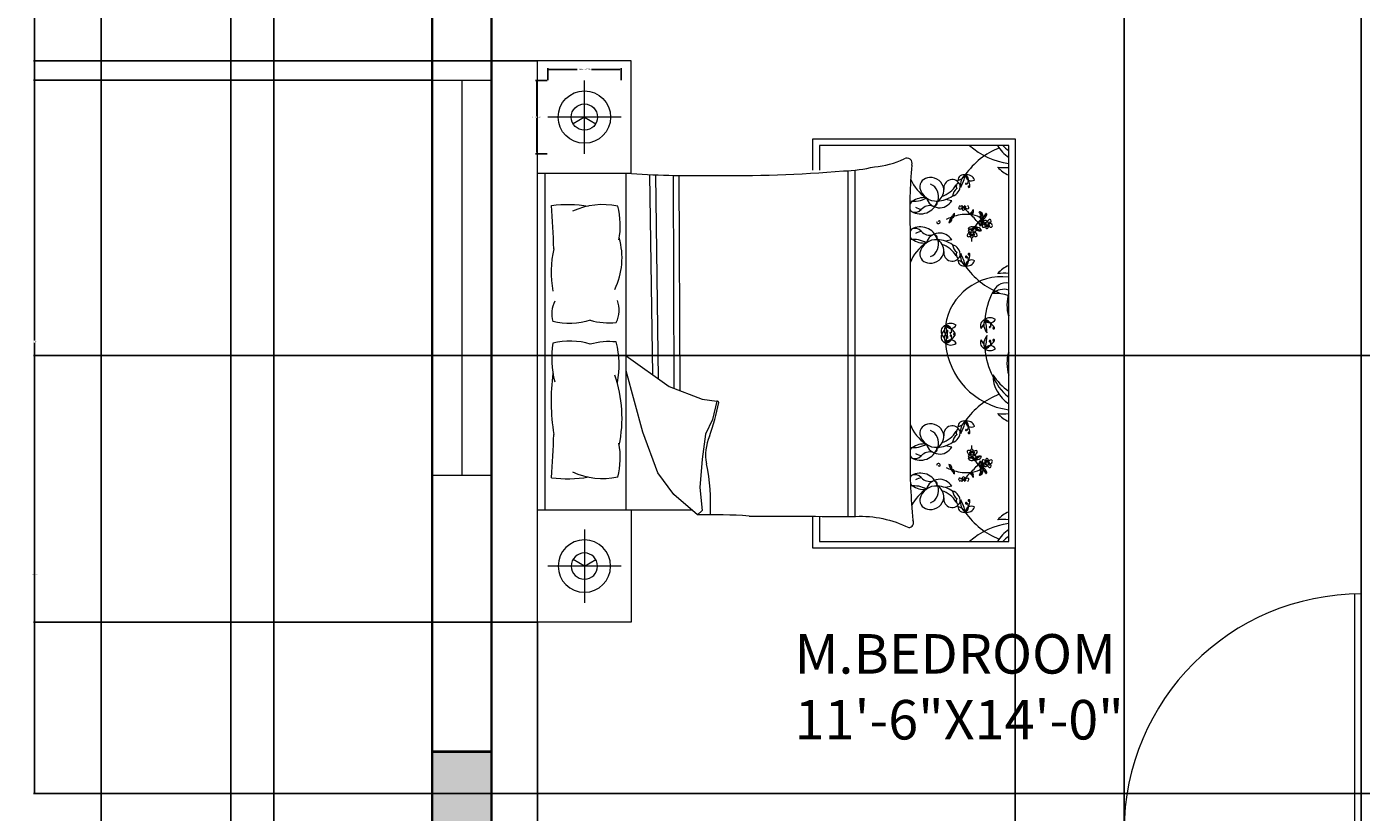
# Model space of a CAD drawing. Units: inches. Extents: x -36 to 401, y -686 to 73.
# Tile 12 of 15: x -36 to 167, y -166 to -47. Entities that reach past the tile are written whole.
import ezdxf

# ---------------------------------------------------------------- set-up
doc = ezdxf.new("R2010")
doc.units = ezdxf.units.IN
doc.header["$MEASUREMENT"] = 0
for name, color, linetype, lineweight in [('A-ANNO-DIMS', 2, 'Continuous', 18), ('A-AREA-IDEN', 7, 'Continuous', 18), ('A-COLS', 7, 'Continuous', 40), ('A-COLS-PATT', 22, 'Continuous', 13), ('A-DOOR', 3, 'Continuous', 18), ('A-FURN', 8, 'Continuous', 13), ('A-GLAZ', 4, 'Continuous', 18), ('A-WALL', 7, 'Continuous', 35), ('C-PROP', 7, 'Continuous', 25)]:
    doc.layers.add(name, color=color, linetype=linetype, lineweight=lineweight)
doc.styles.get("Standard").update_dxf_attribs({"font": 'arial.ttf'})
doc.dimstyles.get("Standard").update_dxf_attribs({"dimtxt": 0.18, "dimasz": 0.18, "dimexe": 0.18, "dimexo": 0.0625, "dimgap": 0.09, "dimtad": 0, "dimtih": 1, "dimtoh": 1, "dimdec": 0, "dimzin": 0, "dimdsep": 46, "dimlunit": 3, "dimtxsty": 'Standard', "dimcen": 0.09, "dimadec": 0, "dimazin": 0, "dimtfac": 1, "dimtdec": 0, "dimtofl": 0, "dimtmove": 0, "dimatfit": 3, "dimfxl": 1, "dimtolj": 1, "dimtzin": 0, "dimarcsym": 0})

# ---------------------------------------------------------------- blocks, each defined once
blk = doc.blocks.new('*D8')
at = {"layer": 'A-ANNO-DIMS', "color": 0, "lineweight": -2, "transparency": 16777216}
for p, q in [((25.63, 7.79), (-24.68, 7.79)), ((-24.5, 7.61), (-24.5, -317.56)), ((-24.5, -649.03), (-24.5, -323.86)), ((1.63, -649.21), (-24.68, -649.21))]:
    blk.add_line(p, q, dxfattribs=at)
at = {"layer": 'A-ANNO-DIMS', "color": 0, "transparency": 16777216}
for points in [[(-24.53, 7.61), (-24.47, 7.61), (-24.5, 7.79)], [(-24.53, -649.03), (-24.47, -649.03), (-24.5, -649.21)]]:
    blk.add_solid(points, dxfattribs=at)
at = {"layer": 'Defpoints', "color": 0, "transparency": 16777216}
for p in [(25.69, 7.79), (-24.5, -649.21), (1.69, -649.21)]:
    blk.add_point(p, dxfattribs=at)
at = {"layer": 'A-ANNO-DIMS', "color": 0, "transparency": 16777216, "insert": (-24.5, -320.71), "char_height": 6, "attachment_point": 5}
blk.add_mtext('\\A1;54\'-9"', dxfattribs=at)
blk = doc.blocks.new('*D11')
at = {"layer": 'A-ANNO-DIMS', "color": 0, "lineweight": -2, "transparency": 16777216}
for p, q in [((25.63, 7.79), (-5.02, 7.79)), ((-4.84, 7.61), (-4.84, -268.06)), ((-4.84, -550.03), (-4.84, -274.36)), ((25.63, -550.21), (-5.02, -550.21))]:
    blk.add_line(p, q, dxfattribs=at)
at = {"layer": 'A-ANNO-DIMS', "color": 0, "transparency": 16777216}
for points in [[(-4.87, 7.61), (-4.81, 7.61), (-4.84, 7.79)], [(-4.87, -550.03), (-4.81, -550.03), (-4.84, -550.21)]]:
    blk.add_solid(points, dxfattribs=at)
at = {"layer": 'Defpoints', "color": 0, "transparency": 16777216}
for p in [(25.69, 7.79), (-4.84, -550.21), (25.69, -550.21)]:
    blk.add_point(p, dxfattribs=at)
at = {"layer": 'A-ANNO-DIMS', "color": 0, "transparency": 16777216, "insert": (-4.84, -271.21), "char_height": 6, "attachment_point": 5}
blk.add_mtext('\\A1;46\'-6"', dxfattribs=at)
blk = doc.blocks.new('WIN-60IN')
for p, q in [((0, 9), (60, 9)), ((0, 0), (0, 9)), ((60, 9), (60, 0)), ((0, 4.5), (60, 4.5)), ((60, 0), (0, 0))]:
    blk.add_line(p, q)
blk = doc.blocks.new('DOOR-SWING-36IN')
for p, q in [((-1, 0), (-1, 36)), ((0, 0), (0, 36))]:
    blk.add_line(p, q)
blk.add_arc((0, 0), 36, 90, 180)
blk = doc.blocks.new('LAMP-BEDSIDE-LARGE')
for p, q in [((5.57, 0), (5.57, 11.14)), ((11.14, 5.57), (0, 5.57))]:
    blk.add_line(p, q)
for points in [[(5.57, 5.57), (3.85, 4.57)], [(5.57, 5.57), (7.29, 4.57)]]:
    blk.add_lwpolyline(points)
for radius in [3.98, 1.99]:
    blk.add_circle((5.57, 5.57), radius)
blk = doc.blocks.new('*D57')
at = {"layer": 'A-ANNO-DIMS', "color": 0, "lineweight": -2, "transparency": 16777216}
for p, q in [((43.24, -55.17), (43.24, -53.38)), ((43.42, -53.56), (47.72, -53.56)), ((54.19, -53.56), (49.89, -53.56)), ((54.37, -55.17), (54.37, -53.38))]:
    blk.add_line(p, q, dxfattribs=at)
at = {"layer": 'A-ANNO-DIMS', "color": 0, "transparency": 16777216}
for points in [[(43.42, -53.53), (43.42, -53.59), (43.24, -53.56)], [(54.19, -53.53), (54.19, -53.59), (54.37, -53.56)]]:
    blk.add_solid(points, dxfattribs=at)
at = {"layer": 'Defpoints', "color": 0, "transparency": 16777216}
for p in [(54.37, -53.56), (43.24, -55.23), (54.37, -55.23)]:
    blk.add_point(p, dxfattribs=at)
at = {"layer": 'A-ANNO-DIMS', "color": 0, "transparency": 16777216, "insert": (48.81, -53.56), "char_height": 0.18, "attachment_point": 5}
blk.add_mtext('\\A1;LAMP 0\'-11" TYP.', dxfattribs=at)
blk = doc.blocks.new('*D58')
at = {"layer": 'A-ANNO-DIMS', "color": 0, "lineweight": -2, "transparency": 16777216}
for p, q in [((43.18, -55.23), (41.39, -55.23)), ((41.57, -55.41), (41.57, -60.62)), ((41.57, -66.19), (41.57, -60.98)), ((43.18, -66.37), (41.39, -66.37))]:
    blk.add_line(p, q, dxfattribs=at)
at = {"layer": 'A-ANNO-DIMS', "color": 0, "transparency": 16777216}
for points in [[(41.54, -55.41), (41.6, -55.41), (41.57, -55.23)], [(41.54, -66.19), (41.6, -66.19), (41.57, -66.37)]]:
    blk.add_solid(points, dxfattribs=at)
at = {"layer": 'Defpoints', "color": 0, "transparency": 16777216}
for p in [(41.57, -55.23), (43.24, -55.23), (43.24, -66.37)]:
    blk.add_point(p, dxfattribs=at)
at = {"layer": 'A-ANNO-DIMS', "color": 0, "transparency": 16777216, "insert": (41.57, -60.8), "char_height": 0.18, "attachment_point": 5}
blk.add_mtext('\\A1;0\'-11" TYP.', dxfattribs=at)
blk = doc.blocks.new('*D68')
at = {"layer": 'A-ANNO-DIMS', "color": 0, "lineweight": -2, "transparency": 16777216}
for p, q in [((25.63, 7.79), (-34.79, 7.79)), ((-34.61, 7.61), (-34.61, -23.53)), ((-34.61, -55.03), (-34.61, -23.89)), ((25.63, -55.21), (-34.79, -55.21))]:
    blk.add_line(p, q, dxfattribs=at)
at = {"layer": 'A-ANNO-DIMS', "color": 0, "transparency": 16777216}
for points in [[(-34.64, 7.61), (-34.58, 7.61), (-34.61, 7.79)], [(-34.64, -55.03), (-34.58, -55.03), (-34.61, -55.21)]]:
    blk.add_solid(points, dxfattribs=at)
at = {"layer": 'Defpoints', "color": 0, "transparency": 16777216}
for p in [(25.69, 7.79), (-34.61, -55.21), (25.69, -55.21)]:
    blk.add_point(p, dxfattribs=at)
at = {"layer": 'A-ANNO-DIMS', "color": 0, "transparency": 16777216, "insert": (-34.61, -23.71), "char_height": 0.18, "attachment_point": 5}
blk.add_mtext('\\A1;5\'-3"', dxfattribs=at)
blk = doc.blocks.new('*D79')
at = {"layer": 'A-ANNO-DIMS', "color": 0, "lineweight": -2, "transparency": 16777216}
for p, q in [((130.69, -398.65), (130.69, 68.27)), ((130.87, 68.09), (148.36, 68.09)), ((166.51, 68.09), (149.02, 68.09)), ((166.69, -398.65), (166.69, 68.27))]:
    blk.add_line(p, q, dxfattribs=at)
at = {"layer": 'A-ANNO-DIMS', "color": 0, "transparency": 16777216}
for points in [[(130.87, 68.12), (130.87, 68.06), (130.69, 68.09)], [(166.51, 68.12), (166.51, 68.06), (166.69, 68.09)]]:
    blk.add_solid(points, dxfattribs=at)
at = {"layer": 'Defpoints', "color": 0, "transparency": 16777216}
for p in [(166.69, 68.09), (130.69, -398.71), (166.69, -398.71)]:
    blk.add_point(p, dxfattribs=at)
at = {"layer": 'A-ANNO-DIMS', "color": 0, "transparency": 16777216, "insert": (148.69, 68.09), "char_height": 0.18, "attachment_point": 5}
blk.add_mtext('\\A1;3\'-0"', dxfattribs=at)
blk = doc.blocks.new('*D85')
at = {"layer": 'A-ANNO-DIMS', "color": 0, "lineweight": -2, "transparency": 16777216}
for p, q in [((114.18, -126.31), (114.18, -685.69)), ((41.7, -137.56), (41.7, -685.69)), ((41.88, -685.51), (77.4, -685.51)), ((114, -685.51), (78.48, -685.51))]:
    blk.add_line(p, q, dxfattribs=at)
at = {"layer": 'A-ANNO-DIMS', "color": 0, "transparency": 16777216}
for points in [[(41.88, -685.48), (41.88, -685.54), (41.7, -685.51)], [(114, -685.48), (114, -685.54), (114.18, -685.51)]]:
    blk.add_solid(points, dxfattribs=at)
at = {"layer": 'Defpoints', "color": 0, "transparency": 16777216}
for p in [(114.18, -126.25), (41.7, -137.5), (114.18, -685.51)]:
    blk.add_point(p, dxfattribs=at)
at = {"layer": 'A-ANNO-DIMS', "color": 0, "transparency": 16777216, "insert": (77.94, -685.51), "char_height": 0.18, "attachment_point": 5}
blk.add_mtext('\\A1;6\'-0 1/2"', dxfattribs=at)
blk = doc.blocks.new('*D86')
at = {"layer": 'A-ANNO-DIMS', "color": 0, "lineweight": -2, "transparency": 16777216}
for p, q in [((41.64, -52.28), (-34.79, -52.28)), ((-34.61, -52.46), (-34.61, -94.71)), ((-34.61, -137.32), (-34.61, -95.07)), ((41.64, -137.5), (-34.79, -137.5))]:
    blk.add_line(p, q, dxfattribs=at)
at = {"layer": 'A-ANNO-DIMS', "color": 0, "transparency": 16777216}
for points in [[(-34.64, -52.46), (-34.58, -52.46), (-34.61, -52.28)], [(-34.64, -137.32), (-34.58, -137.32), (-34.61, -137.5)]]:
    blk.add_solid(points, dxfattribs=at)
at = {"layer": 'Defpoints', "color": 0, "transparency": 16777216}
for p in [(41.7, -52.28), (-34.61, -137.5), (41.7, -137.5)]:
    blk.add_point(p, dxfattribs=at)
at = {"layer": 'A-ANNO-DIMS', "color": 0, "transparency": 16777216, "insert": (-34.61, -94.89), "char_height": 0.18, "attachment_point": 5}
blk.add_mtext('\\A1;7\'-1"', dxfattribs=at)
blk = doc.blocks.new('*D88')
at = {"layer": 'A-ANNO-DIMS', "color": 0, "lineweight": -2, "transparency": 16777216}
for p, q in [((187.04, -96.98), (-34.79, -96.98)), ((-34.61, -97.16), (-34.61, -130.08)), ((-34.61, -163.35), (-34.61, -130.44)), ((187.04, -163.53), (-34.79, -163.53))]:
    blk.add_line(p, q, dxfattribs=at)
at = {"layer": 'A-ANNO-DIMS', "color": 0, "transparency": 16777216}
for points in [[(-34.64, -97.16), (-34.58, -97.16), (-34.61, -96.98)], [(-34.64, -163.35), (-34.58, -163.35), (-34.61, -163.53)]]:
    blk.add_solid(points, dxfattribs=at)
at = {"layer": 'Defpoints', "color": 0, "transparency": 16777216}
for p in [(187.11, -96.98), (-34.61, -163.53), (187.11, -163.53)]:
    blk.add_point(p, dxfattribs=at)
at = {"layer": 'A-ANNO-DIMS', "color": 0, "transparency": 16777216, "insert": (-34.61, -130.26), "char_height": 0.18, "attachment_point": 5}
blk.add_mtext('\\A1;5\'-6 1/2"', dxfattribs=at)

msp = doc.modelspace()

# ---------------------------------------------------------------- hatches: boundary and pattern name
at = {"layer": 'A-COLS-PATT'}
h = msp.add_hatch(color=256, dxfattribs=at)
h.dxf.hatch_style = 1
h.paths.add_polyline_path([(34.69, 7.79), (25.69, 7.79), (25.69, -13.21), (34.69, -13.21)])
h.paths.add_polyline_path([(172.69, -13.21), (177.19, -13.21), (181.69, -13.21), (181.69, 7.79), (172.69, 7.79)])
h.paths.add_polyline_path([(322.69, 7.79), (313.69, 7.79), (313.69, -13.21), (322.69, -13.21)])
h.paths.add_polyline_path([(322.69, -157.21), (313.69, -157.21), (313.69, -178.21), (322.69, -178.21)])
h.paths.add_polyline_path([(172.69, -178.21), (177.19, -178.21), (181.69, -178.21), (181.69, -157.21), (177.19, -157.21), (172.69, -157.21)])
h.paths.add_polyline_path([(25.69, -178.21), (34.69, -178.21), (34.69, -157.21), (25.69, -157.21)])
h.paths.add_polyline_path([(34.69, -325.21), (25.69, -325.21), (25.69, -346.21), (34.69, -346.21)])
h.paths.add_polyline_path([(181.69, -325.21), (177.19, -325.21), (172.69, -325.21), (172.69, -346.21), (177.19, -346.21), (181.69, -346.21)])
h.paths.add_polyline_path([(322.69, -325.21), (313.69, -325.21), (313.69, -346.21), (322.69, -346.21)])
h.paths.add_polyline_path([(364.69, -451.21), (358.69, -451.21), (358.69, -472.21), (364.69, -472.21)])
h.paths.add_polyline_path([(181.69, -451.21), (177.19, -451.21), (172.69, -451.21), (172.69, -472.21), (177.19, -472.21), (181.69, -472.21)])
h.paths.add_polyline_path([(25.69, -472.21), (34.69, -472.21), (34.69, -451.21), (25.69, -451.21)])

# ---------------------------------------------------------------- linework, layer by layer
at = {"layer": 'A-COLS'}
msp.add_line((34.69, -157.21), (25.69, -157.21), dxfattribs=at)
at = {"layer": 'A-FURN'}
for p, q in [((41.7, -137.5), (41.7, -52.28)), ((83.48, -68.85), (83.48, -64.12)), ((83.48, -64.12), (114.18, -64.12)), ((114.18, -64.12), (114.18, -126.25)), ((84.47, -65.11), (84.47, -68.86)), ((113.19, -65.11), (84.47, -65.11)), ((113.19, -125.26), (113.19, -65.11)), ((42.8, -69.32), (42.8, -120.45)), ((55.17, -120.45), (55.17, -69.32)), ((58.71, -69.55), (59.14, -99.89)), ((59.59, -69.58), (60.02, -100.53)), ((62.27, -69.63), (62.4, -101.99)), ((63.14, -69.62), (63.28, -102.32)), ((88.79, -68.93), (88.79, -121.43)), ((89.86, -68.85), (89.86, -121.43)), ((104.55, -73.51), (103.59, -73.32)), ((98.23, -77.59), (98.23, -112.19)), ((104.55, -79.46), (103.59, -79.65)), ((55.17, -97.04), (61.67, -101.71)), ((57.7, -108.62), (55.17, -99.32)), ((61.67, -101.71), (66.67, -103.61)), ((66.67, -103.61), (68.92, -103.96)), ((68.92, -103.96), (68.23, -106.72)), ((68.23, -106.72), (67.19, -108.96)), ((59.95, -114.83), (57.7, -108.62)), ((67.19, -108.96), (66.67, -112.76)), ((104.55, -110.91), (103.59, -110.72)), ((66.67, -112.76), (66.33, -117.07)), ((62.36, -118.11), (59.95, -114.83)), ((66.33, -117.07), (66.67, -120.53)), ((104.55, -116.86), (103.59, -117.05)), ((65.98, -121.22), (62.36, -118.11)), ((41.7, -120.45), (65.09, -120.45)), ((66.67, -120.53), (65.98, -121.22)), ((83.48, -126.25), (83.48, -121.43)), ((84.47, -121.43), (84.47, -125.26)), ((84.47, -125.26), (113.19, -125.26)), ((114.18, -126.25), (83.48, -126.25))]:
    msp.add_line(p, q, dxfattribs=at)
for points in [[(41.7, -69.32), (55.91, -69.32), (55.91, -52.28), (41.7, -52.28)], [(55.91, -120.45), (55.91, -137.5), (41.7, -137.5)]]:
    msp.add_lwpolyline(points, dxfattribs=at)
for points in [[(88.12, -68.96, 0.056112), (92.81, -68.34, 0.095341), (97.33, -67.14)], [(43.83, -74.22, -0.074897), (49.39, -74.32, 0.472817)], [(49.71, -91.65, -0.14099), (44.03, -91.82, -0.235245)], [(49.71, -95.29, 0.14099), (44.03, -95.12, 0.235245)], [(43.83, -115.56, 0.074897), (49.39, -115.45, -0.472817)], [(73.79, -121.39, 0.001242), (89.96, -121.43, -0.127202), (98.02, -123.14)]]:
    msp.add_lwpolyline(points, format="xyb", dxfattribs=at)
for centre in [(109.93, -77.01), (107.64, -78.43), (107.64, -111.94), (109.93, -113.36)]:
    msp.add_circle(centre, 0.217, dxfattribs=at)
for centre, radius, start, end in [((115.79, -75.86), 11.13, 111.4092, 145.6135), ((114.69, -56.82), 11.13, 228.1144, 262.255), ((116.18, -62.4), 5.42, 209.8884, 236.5383), ((117.19, -60.45), 6.76, 223.5186, 233.6964), ((97.76, -67.79), 0.777, 336.5219, 123.8264), ((181.11, -74.98), 82.93, 175.2402, 181.8035), ((114.93, -65.44), 4.52, 221.0454, 247.4453), ((112.49, -53.05), 15.4, 266.3481, 272.5919), ((65.59, 83.45), 153.13, 266.1, 270.9282), ((71.15, 130.07), 199.75, 269.1145, 274.8735), ((104.23, -67.68), 6.45, 203.6453, 236.3329), ((101.13, -71.43), 1.44, 88.9462, 185.5144), ((101.34, -72.02), 2.04, 7.1143, 95.0551), ((104.62, -71.56), 1.28, 19.1312, 189.736), ((106.01, -71.29), 0.784, 126.7319, 206.0245), ((106.39, -70.47), 0.923, 76.272, 177.0484), ((104.98, -68.59), 1.9, 284.7031, 328.6173), ((107.64, -71), 1.76, 125.7657, 194.5347), ((99.01, -67.89), 7.79, 332.8176, 347.4827), ((106.87, -70.78), 1.23, 20.9613, 102.2885), ((107.54, -69.55), 0.929, 181.7131, 301.5367), ((104.49, -71.43), 2.81, 2.0648, 41.1598), ((106.18, -70.38), 0.91, 316.2238, 62.3173), ((106.71, -70.92), 0.0725, 20.2667, 316.2271), ((102.2, -70.99), 2.56, 193.079, 274.7067), ((100.57, -72.82), 1.98, 338.5779, 68.4181), ((100.89, -71.67), 2.48, 305.9599, 357.6409), ((102.13, -68.98), 4.57, 273.4924, 303.7117), ((101.8, -69.02), 4.02, 288.2955, 328.7386), ((104.23, -71.25), 1.6, 285.6955, 4.031), ((106.36, -72.97), 1.7, 128.4175, 173.8338), ((107.16, -71.33), 0.138, 168.5166, 2.0648), ((107.09, -71.32), 0.0671, 52.0591, 168.5166), ((-767.19, -121.19), 812.38, 2.85022, 3.31479), ((51.63, -85.07), 10.98, 78.2417, 114.8684), ((42.83, -77.26), 11.42, 348.9631, 14.8961), ((99.17, -74.42), 1.03, 127.675, 162.5814), ((99.17, -74.42), 1.03, 196.6343, 225.5483), ((98.86, -70.04), 3.53, 259.249, 301.1782), ((99.78, -72.78), 2.72, 240.8249, 340.7178), ((98.97, -73.98), 1.28, 246.1646, 318.4347), ((100.39, -76.32), 3.29, 85.2696, 124.215), ((100.27, -72.37), 2.45, 240.0851, 262.564), ((101.23, -75.99), 1.75, 74.8529, 138.4347), ((102.71, -72.45), 2.12, 196.8663, 330.0915), ((101.82, -73.79), 0.529, 254.8529, 12.6959), ((100.39, -76.32), 3.29, 53.6555, 57.2989), ((105.75, -74.59), 0.168, 125.0752, 284.7644), ((106.01, -74.52), 0.362, 127.3642, 168.4363), ((105.73, -74.23), 0.522, 277.4968, 341.2737), ((106.14, -74.47), 0.207, 88.1325, 178.8919), ((106.56, -74.69), 0.449, 136.3462, 189.6513), ((106.3, -74.74), 0.187, 189.6513, 312.3208), ((106.35, -74.22), 0.217, 183.2768, 356.7232), ((107.03, -74.61), 0.71, 164.2829, 186.9148), ((106.19, -74.61), 0.355, 312.3208, 40.2111), ((106.94, -74.21), 0.504, 201.6382, 274.947), ((106.27, -74.9), 0.659, 42.3896, 66.5724), ((112.92, -69.69), 8.09, 217.9541, 226.8459), ((106.75, -74.52), 0.358, 10.9597, 52.2379), ((106.97, -74.55), 0.167, 274.947, 37.5263), ((108.03, -75.28), 0.447, 115.5379, 168.6744), ((106.51, -74.64), 1.35, 329.344, 349.7412), ((105.44, -74.95), 2.4, 352.8698, 1.6736), ((102.52, -76.71), 0.267, 169.5864, 349.5616), ((102.63, -76.73), 0.164, 349.5616, 167.2949), ((106.92, -82.63), 7.06, 110.1059, 116.9968), ((104.55, -76.82), 0.447, 129.5056, 182.6421), ((103.26, -75.78), 1.35, 308.4388, 328.836), ((103.03, -74.69), 2.4, 296.5064, 305.3102), ((103.01, -75.92), 1.37, 336.3901, 344.4871), ((104.5, -76.27), 0.174, 83.9457, 185.6216), ((103.8, -76.11), 0.714, 328.836, 0.8141), ((104.17, -76.32), 0.409, 306.5232, 32.4668), ((104.66, -76), 0.174, 112.5583, 214.2343), ((104.55, -75.69), 0.409, 265.7131, 351.6568), ((104.19, -75.47), 0.714, 297.3659, 329.344), ((103.65, -74.85), 1.37, 313.6929, 321.7899), ((105.16, -75.79), 0.447, 115.5379, 168.6744), ((103.65, -75.14), 1.35, 329.344, 349.7412), ((106.92, -82.63), 7.06, 86.1723, 106.4158), ((102.57, -75.45), 2.4, 352.8698, 1.6736), ((107.53, -75.49), 0.174, 112.5583, 214.2343), ((107.42, -75.18), 0.409, 265.7131, 351.6568), ((107.06, -74.96), 0.714, 297.3659, 329.344), ((107.09, -79.12), 3.54, 60.7959, 85.244), ((99.56, -84.21), 11.64, 37.8256, 47.7588), ((106.52, -74.34), 1.37, 313.6929, 321.7899), ((111.79, -79.48), 4.24, 130.182, 149.456), ((108.82, -75.43), 0.242, 33.0979, 123.1364), ((103.48, -78.85), 6.34, 31.1156, 34.8118), ((108.47, -75.85), 0.656, 2.3172, 70.5201), ((109.46, -77.06), 0.7, 139.3812, 199.9959), ((108.15, -76.56), 0.989, 310.9365, 22.7695), ((108.6, -76.61), 0.719, 285.6484, 332.2957), ((109.01, -76.01), 0.189, 135.7354, 318.1297), ((108.69, -75.7), 0.251, 315.7354, 31.1156), ((108.48, -76.23), 0.582, 319.3812, 5.5456), ((109.15, -76.01), 0.189, 68.2452, 250.6395), ((108.71, -75.77), 0.565, 352.6008, 57.1845), ((110.73, -79.57), 3.78, 111.7087, 116.2181), ((107.09, -79.12), 3.54, 47.5083, 55.9967), ((109.25, -75.64), 0.565, 252.8042, 349.6943), ((108.71, -76.66), 0.601, 331.1838, 51.6792), ((109.31, -75.6), 0.251, 248.2452, 323.6254), ((109.59, -77.31), 0.362, 93.635, 168.4363), ((109.09, -75.44), 0.656, 291.7087, 3.0299), ((109.54, -76.74), 0.213, 138.2946, 276.2474), ((109.62, -76.77), 0.296, 358.5719, 143.8954), ((104.41, -71.99), 6.34, 323.6254, 327.3216), ((109.8, -76.54), 0.299, 208.8493, 269.9355), ((109.54, -76.61), 0.341, 274.2123, 318.1587), ((109.61, -75.61), 0.242, 325.6077, 55.6462), ((110.58, -76.95), 0.684, 121.9501, 165.2442), ((110.11, -76.69), 0.144, 262.868, 7.094), ((110.09, -76.57), 0.428, 278.5614, 22.5914), ((110.33, -77.3), 0.358, 10.9597, 118.7804), ((110.33, -76.55), 0.215, 44.3732, 121.9501), ((99.17, -78.55), 1.03, 134.4517, 156.7144), ((99.17, -78.55), 1.03, 203.2856, 232.325), ((99.78, -80.19), 2.72, 19.2822, 119.1751), ((98.97, -78.98), 1.28, 41.5653, 113.8354), ((100.27, -80.6), 2.45, 97.436, 119.9149), ((101.23, -76.98), 1.75, 221.5653, 285.1471), ((102.71, -80.52), 2.12, 29.9085, 163.1337), ((101.82, -79.18), 0.529, 347.3041, 105.1471), ((107.04, -78.79), 0.168, 125.0752, 284.7644), ((107.3, -78.73), 0.362, 93.635, 168.4363), ((107.32, -76.77), 0.989, 253.6301, 325.4631), ((107.59, -78.14), 0.7, 82.0748, 142.6895), ((107.52, -77.18), 0.719, 228.342, 274.9894), ((107.26, -78.16), 0.213, 138.2946, 276.2474), ((107.02, -78.44), 0.522, 277.4968, 341.2737), ((107.34, -78.19), 0.296, 358.5719, 143.8954), ((107.43, -78.68), 0.207, 88.1325, 178.8919), ((107.51, -77.96), 0.299, 208.8493, 269.9355), ((107.25, -78.03), 0.341, 274.2123, 318.1587), ((107.85, -78.9), 0.449, 136.3462, 189.6513), ((107.54, -77.3), 0.601, 273.8774, 357.1501), ((108.32, -78.82), 0.71, 164.2829, 186.9148), ((108.29, -78.37), 0.684, 121.9501, 165.2442), ((107.77, -76.87), 0.582, 262.0748, 308.2393), ((107.48, -78.82), 0.355, 312.3208, 40.2111), ((108.23, -78.42), 0.504, 201.6382, 274.947), ((107.82, -78.11), 0.144, 262.868, 7.094), ((107.56, -79.11), 0.659, 42.3896, 66.5724), ((107.8, -77.99), 0.428, 278.5614, 22.5914), ((108.04, -78.72), 0.358, 10.9597, 118.7804), ((111.79, -79.48), 4.24, 156.1523, 156.9499), ((108.05, -77.97), 0.215, 44.3732, 121.9501), ((108.71, -77.47), 0.601, 181.4625, 249.4747), ((108.61, -76.99), 0.582, 215.1128, 261.2773), ((109.07, -77.02), 0.989, 197.889, 269.722), ((108.26, -78.76), 0.167, 274.947, 37.5263), ((108.76, -77.36), 0.719, 248.3627, 295.0101), ((108.41, -78.26), 0.7, 20.6625, 81.2773), ((109.33, -77.37), 0.168, 125.0752, 284.7644), ((109.31, -77.02), 0.522, 277.4968, 341.2737), ((109.72, -77.26), 0.207, 88.1325, 178.8919), ((110.14, -77.48), 0.449, 136.3462, 189.6513), ((109.88, -77.53), 0.187, 189.6513, 312.3208), ((110.6, -77.4), 0.71, 164.2829, 186.9148), ((109.77, -77.4), 0.355, 312.3208, 40.2111), ((110.52, -77), 0.504, 201.6382, 274.947), ((109.85, -77.69), 0.659, 42.3896, 66.5724), ((110.55, -77.34), 0.167, 274.947, 37.5263), ((58.74, -84.33), 14.98, 166.3427, 191.1841), ((43.67, -82.18), 10.85, 333.8761, 16.1746), ((98.86, -82.92), 3.53, 58.8218, 100.2867), ((104.23, -85.29), 6.45, 123.6671, 158.5059), ((100.39, -76.64), 3.29, 235.785, 274.7304), ((102.2, -81.97), 2.56, 85.2933, 166.921), ((100.57, -80.14), 1.98, 291.5819, 21.4221), ((100.39, -76.64), 3.29, 302.7011, 306.3445), ((100.89, -81.3), 2.48, 2.3591, 54.0401), ((102.13, -83.98), 4.57, 56.2883, 86.5076), ((101.8, -83.95), 4.02, 31.2614, 71.7045), ((106.36, -80), 1.7, 186.1662, 231.5825), ((104.23, -81.72), 1.6, 355.969, 74.3045), ((107.59, -78.95), 0.187, 189.6513, 312.3208), ((111.79, -79.48), 4.24, 175.2415, 182.8929), ((101.13, -81.53), 1.44, 174.4856, 271.0538), ((101.34, -80.94), 2.04, 264.9449, 352.8857), ((104.62, -81.41), 1.28, 170.264, 340.8688), ((106.01, -81.67), 0.784, 153.9755, 233.2681), ((106.39, -82.49), 0.923, 182.9516, 283.728), ((104.98, -84.38), 1.9, 31.3827, 75.2969), ((107.64, -81.96), 1.76, 165.4653, 234.2343), ((99.01, -85.08), 7.79, 12.5173, 27.1824), ((104.49, -81.54), 2.81, 318.8402, 357.9352), ((106.18, -82.58), 0.91, 297.6827, 43.7762), ((107.54, -83.42), 0.929, 58.4633, 178.2869), ((106.87, -82.18), 1.23, 257.7115, 339.0387), ((106.75, -82.04), 0.12, 43.7762, 339.7183), ((107.16, -81.63), 0.138, 357.9352, 191.4834), ((107.09, -81.65), 0.0671, 191.4834, 307.9409), ((115.79, -77.1), 11.13, 214.3865, 248.5908), ((114.93, -87.52), 4.52, 112.5547, 138.9546), ((112.49, -99.92), 15.4, 87.4081, 93.6519), ((112.12, -93.66), 8.61, 82.8636, 171.8197), ((112.72, -87.98), 2, 76.3898, 169.0739), ((112.45, -89.48), 2.53, 72.8609, 131.9049), ((48.08, -90.65), 4.22, 153.3437, 196.1026), ((49.55, -90.08), 4.52, 335.0183, 18.5407), ((120.65, -92.45), 11.13, 152.5854, 175.5377), ((111.33, -92.55), 4.98, 68.117, 96.6195), ((119.04, -89.34), 6.12, 162.9798, 196.4569), ((122.2, -91.76), 9.05, 174.3643, 175.6213), ((128.4, -96.53), 16.17, 160.0972, 160.2783), ((52.55, -81.6), 10.44, 254.1707, 275.9871), ((103.85, -93.32), 0.923, 106.1963, 206.9726), ((101.7, -92.39), 1.9, 314.6273, 358.5415), ((105.2, -93.16), 1.76, 155.6899, 224.4589), ((105.2, -94.37), 1.76, 135.5411, 204.3101), ((104.42, -93.35), 1.23, 50.8855, 132.2127), ((104.39, -91.95), 0.929, 211.6373, 331.4609), ((103.63, -93.35), 0.91, 346.148, 92.2415), ((102.68, -95.1), 2.81, 31.989, 71.0841), ((96.17, -94.77), 7.79, 2.7418, 17.407), ((96.17, -92.76), 7.79, 342.593, 357.2582), ((109.81, -92.47), 0.923, 106.1963, 206.9726), ((107.66, -91.54), 1.9, 314.6273, 358.5415), ((111.16, -92.31), 1.76, 155.6899, 224.4589), ((110.39, -92.5), 1.23, 50.8855, 132.2127), ((110.35, -91.1), 0.929, 211.6373, 331.4609), ((109.59, -92.5), 0.91, 346.148, 92.2415), ((108.64, -94.25), 2.81, 31.989, 71.0841), ((102.13, -93.91), 7.79, 2.7418, 17.407), ((110.31, -92.7), 0.0725, 50.1909, 346.0209), ((110.91, -92.83), 0.138, 198.4408, 31.989), ((110.85, -92.85), 0.0671, 81.9833, 198.4408), ((59.05, -97.35), 15.19, 171.5249, 193.96), ((52.55, -105.33), 10.44, 84.0129, 105.8293), ((39.04, -98.49), 15.03, 349.8617, 13.6238), ((103.85, -94.2), 0.923, 153.0274, 253.8037), ((101.7, -95.14), 1.9, 1.4585, 45.3727), ((102.68, -92.43), 2.81, 288.9159, 328.011), ((103.63, -94.18), 0.91, 267.7585, 13.852), ((104.39, -95.58), 0.929, 28.5391, 148.3627), ((104.42, -94.18), 1.23, 227.7873, 309.1145), ((114.69, -94.22), 11.13, 184.4623, 262.255), ((104.35, -93.55), 0.0725, 50.1909, 346.0209), ((104.4, -93.99), 0.12, 13.852, 309.9245), ((104.95, -93.68), 0.138, 198.4408, 31.989), ((104.89, -93.7), 0.0671, 81.9833, 198.4408), ((104.95, -93.85), 0.138, 328.011, 161.5592), ((104.89, -93.82), 0.0671, 161.5592, 278.0167), ((109.81, -95.06), 0.923, 153.0274, 253.8037), ((107.66, -95.99), 1.9, 1.4585, 45.3727), ((111.16, -95.22), 1.76, 135.5411, 204.3101), ((102.13, -93.61), 7.79, 342.593, 357.2582), ((108.64, -93.28), 2.81, 288.9159, 328.011), ((109.59, -95.03), 0.91, 267.7585, 13.852), ((110.36, -94.84), 0.12, 13.852, 309.9245), ((110.91, -94.7), 0.138, 328.011, 161.5592), ((110.85, -94.67), 0.0671, 161.5592, 278.0167), ((110.35, -96.43), 0.929, 28.5391, 148.3627), ((110.39, -95.03), 1.23, 227.7873, 309.1145), ((120.65, -95.08), 11.13, 184.4623, 207.4146), ((119.04, -98.19), 6.12, 163.5431, 197.0202), ((122.2, -95.76), 9.05, 184.3787, 185.6357), ((128.4, -91), 16.17, 199.7217, 199.9028), ((74.67, -103.88), 30.91, 172.2196, 189.497), ((34.71, -106.51), 19.81, 348.0397, 19.2615), ((116.18, -99.81), 5.42, 181.272, 236.5383), ((119.09, -94.3), 10.05, 214.0123, 234.053), ((117.19, -97.86), 6.76, 197.8504, 233.6964), ((115.79, -113.26), 11.13, 111.4092, 145.6135), ((36.71, -98.04), 33.05, 340.1194, 349.3383), ((68.99, -104.15), 0.206, 358.8623, 109.7536), ((106.39, -107.87), 0.923, 76.272, 177.0484), ((104.98, -105.99), 1.9, 284.7031, 328.6173), ((107.64, -108.41), 1.76, 125.7657, 194.5347), ((99.01, -105.29), 7.79, 332.8176, 347.4827), ((106.87, -108.18), 1.23, 20.9613, 102.2885), ((106.18, -107.78), 0.91, 316.2238, 62.3173), ((104.49, -108.83), 2.81, 2.0648, 41.1598), ((107.54, -106.95), 0.929, 181.7131, 301.5367), ((112.49, -90.45), 15.4, 266.3481, 272.5919), ((114.93, -102.84), 4.52, 221.0454, 247.4453), ((-767.19, -68.59), 812.38, 356.68521, 357.14978), ((74.14, -112.07), 6.94, 156.2616, 191.3392), ((104.23, -105.08), 6.45, 201.4941, 236.3329), ((101.13, -108.84), 1.44, 88.9462, 185.5144), ((102.2, -108.39), 2.56, 193.079, 274.7067), ((101.34, -109.43), 2.04, 7.1143, 95.0551), ((100.57, -110.23), 1.98, 338.5779, 68.4181), ((100.89, -109.07), 2.48, 305.9599, 357.6409), ((101.8, -106.42), 4.02, 288.2955, 328.7386), ((104.62, -108.96), 1.28, 19.1312, 189.736), ((104.23, -108.65), 1.6, 285.6955, 4.031), ((106.36, -110.37), 1.7, 128.4175, 173.8338), ((106.01, -108.69), 0.784, 126.7319, 206.0245), ((106.71, -108.32), 0.0725, 20.2667, 316.2271), ((107.16, -108.73), 0.138, 168.5166, 2.0648), ((107.09, -108.72), 0.0671, 52.0591, 168.5166), ((42.83, -112.52), 11.42, 345.1039, 11.0369), ((98.86, -107.44), 3.53, 259.7133, 301.1782), ((99.17, -111.82), 1.03, 127.675, 156.7144), ((99.78, -110.18), 2.72, 240.8249, 340.7178), ((100.39, -113.72), 3.29, 85.2696, 124.215), ((102.71, -109.85), 2.12, 196.8663, 330.0915), ((101.82, -111.19), 0.529, 254.8529, 12.6959), ((100.39, -113.72), 3.29, 53.6555, 57.2989), ((102.13, -106.38), 4.57, 273.4924, 303.7117), ((107.59, -111.42), 0.187, 47.6792, 170.3487), ((111.79, -110.89), 4.24, 177.1071, 184.7585), ((107.48, -111.55), 0.355, 319.7889, 47.6792), ((186.94, -113.2), 88.72, 179.3433, 185.6887), ((99.17, -111.82), 1.03, 203.229, 225.5483), ((98.97, -111.38), 1.28, 246.1646, 318.4347), ((100.27, -109.77), 2.45, 240.0851, 262.564), ((101.23, -113.39), 1.75, 74.8529, 138.4347), ((102.52, -113.66), 0.267, 10.4384, 190.4136), ((107.04, -111.58), 0.168, 75.2356, 234.9248), ((107.3, -111.64), 0.362, 191.5637, 266.365), ((107.26, -112.21), 0.213, 83.7526, 221.7054), ((107.52, -113.19), 0.719, 85.0106, 131.658), ((107.32, -113.6), 0.989, 34.5369, 106.3699), ((107.59, -112.23), 0.7, 217.3105, 277.9252), ((107.02, -111.93), 0.522, 18.7263, 82.5032), ((107.34, -112.18), 0.296, 216.1046, 1.4281), ((107.43, -111.69), 0.207, 181.1081, 271.8675), ((107.51, -112.41), 0.299, 90.0645, 151.1507), ((107.25, -112.34), 0.341, 41.8413, 85.7877), ((99.56, -106.16), 11.64, 312.2412, 322.1744), ((107.85, -111.47), 0.449, 170.3487, 223.6538), ((107.54, -113.07), 0.601, 2.8499, 86.1226), ((108.32, -111.55), 0.71, 173.0852, 195.7171), ((108.29, -112), 0.684, 194.7558, 238.0499), ((107.77, -113.5), 0.582, 51.7607, 97.9252), ((108.23, -111.95), 0.504, 85.053, 158.3618), ((107.82, -112.26), 0.144, 352.906, 97.132), ((107.56, -111.26), 0.659, 293.4276, 317.6104), ((108.04, -111.64), 0.358, 241.2196, 349.0403), ((107.8, -112.38), 0.428, 337.4086, 81.4386), ((111.79, -110.89), 4.24, 203.0501, 203.8477), ((108.05, -112.4), 0.215, 238.0499, 315.6268), ((108.71, -112.9), 0.601, 110.5253, 178.5375), ((109.07, -113.34), 0.989, 90.278, 162.111), ((108.61, -113.38), 0.582, 98.7227, 144.8872), ((111.79, -110.89), 4.24, 210.544, 229.818), ((108.26, -111.61), 0.167, 322.4737, 85.053), ((108.76, -113.01), 0.719, 64.9899, 111.6373), ((108.41, -112.11), 0.7, 278.7227, 339.3375), ((109.46, -113.3), 0.7, 160.0041, 220.6188), ((108.15, -113.81), 0.989, 337.2305, 49.0635), ((108.6, -113.76), 0.719, 27.7043, 74.3516), ((109.33, -112.99), 0.168, 75.2356, 234.9248), ((109.59, -113.06), 0.362, 191.5637, 266.365), ((109.31, -113.35), 0.522, 18.7263, 82.5032), ((109.72, -113.11), 0.207, 181.1081, 271.8675), ((110.14, -112.89), 0.449, 170.3487, 223.6538), ((109.88, -112.84), 0.187, 47.6792, 170.3487), ((110.6, -112.97), 0.71, 173.0852, 195.7171), ((109.77, -112.97), 0.355, 319.7889, 47.6792), ((110.52, -113.37), 0.504, 85.053, 158.3618), ((109.85, -112.68), 0.659, 293.4276, 317.6104), ((110.33, -113.06), 0.358, 241.2196, 349.0403), ((110.09, -113.8), 0.428, 337.4086, 81.4386), ((110.55, -113.03), 0.167, 322.4737, 85.053), ((51.63, -104.7), 10.98, 245.1316, 281.7583), ((35.81, -119.76), 32.16, 357.4519, 11.3392), ((99.17, -115.95), 1.03, 134.4517, 153.558), ((99.78, -117.59), 2.72, 19.2822, 119.1751), ((98.97, -116.39), 1.28, 41.5653, 113.8354), ((102.63, -113.64), 0.164, 192.7051, 10.4384), ((106.92, -107.73), 7.06, 243.0032, 249.8941), ((103.26, -114.59), 1.35, 31.164, 51.5612), ((104.55, -113.55), 0.447, 177.3579, 230.4944), ((103.03, -115.68), 2.4, 54.6898, 63.4936), ((103.01, -114.45), 1.37, 15.5129, 23.6099), ((104.5, -114.1), 0.174, 174.3784, 276.0543), ((104.17, -114.05), 0.409, 327.5332, 53.4768), ((103.8, -114.26), 0.714, 359.1859, 31.164), ((104.66, -114.37), 0.174, 145.7657, 247.4417), ((104.55, -114.68), 0.409, 8.3432, 94.2869), ((104.19, -114.9), 0.714, 30.656, 62.6341), ((103.65, -115.52), 1.37, 38.2101, 46.3071), ((105.16, -114.58), 0.447, 191.3256, 244.4621), ((103.65, -115.23), 1.35, 10.2588, 30.656), ((106.92, -107.73), 7.06, 253.5842, 273.8277), ((102.57, -114.92), 2.4, 358.3264, 7.1302), ((112.92, -120.68), 8.09, 133.1541, 142.0459), ((107.53, -114.87), 0.174, 145.7657, 247.4417), ((107.09, -111.25), 3.54, 274.756, 299.2041), ((107.42, -115.18), 0.409, 8.3432, 94.2869), ((107.06, -115.41), 0.714, 30.656, 62.6341), ((106.52, -116.02), 1.37, 38.2101, 46.3071), ((108.03, -115.09), 0.447, 191.3256, 244.4621), ((106.51, -115.73), 1.35, 10.2588, 30.656), ((105.44, -115.42), 2.4, 358.3264, 7.1302), ((108.47, -114.52), 0.656, 289.4799, 357.6828), ((103.48, -111.52), 6.34, 325.1882, 328.8844), ((108.82, -114.94), 0.242, 236.8636, 326.9021), ((109.01, -114.36), 0.189, 41.8703, 224.2646), ((108.69, -114.67), 0.251, 328.8844, 44.2646), ((108.48, -114.14), 0.582, 354.4544, 40.6188), ((109.15, -114.36), 0.189, 109.3605, 291.7548), ((108.71, -114.6), 0.565, 302.8155, 7.3992), ((110.73, -110.8), 3.78, 243.7819, 248.2913), ((107.09, -111.25), 3.54, 304.0033, 312.4917), ((108.71, -113.71), 0.601, 308.3208, 28.8162), ((109.25, -114.72), 0.565, 10.3057, 107.1958), ((109.31, -114.77), 0.251, 36.3746, 111.7548), ((109.54, -113.63), 0.213, 83.7526, 221.7054), ((109.09, -114.92), 0.656, 356.9701, 68.2913), ((109.62, -113.6), 0.296, 216.1046, 1.4281), ((104.41, -118.38), 6.34, 32.6784, 36.3746), ((109.8, -113.83), 0.299, 90.0645, 151.1507), ((109.54, -113.76), 0.341, 41.8413, 85.7877), ((109.61, -114.76), 0.242, 304.3538, 34.3923), ((110.58, -113.42), 0.684, 194.7558, 238.0499), ((110.11, -113.68), 0.144, 352.906, 97.132), ((110.33, -113.82), 0.215, 238.0499, 315.6268), ((99.17, -115.95), 1.03, 210.0293, 232.325), ((98.86, -120.33), 3.53, 58.8218, 99.1554), ((104.23, -122.69), 6.45, 123.6671, 153.2997), ((100.39, -114.05), 3.29, 235.785, 274.7304), ((100.27, -118), 2.45, 97.436, 119.9149), ((102.2, -119.38), 2.56, 85.2933, 166.921), ((101.23, -114.38), 1.75, 221.5653, 285.1471), ((102.71, -117.92), 2.12, 29.9085, 163.1337), ((100.57, -117.54), 1.98, 291.5819, 21.4221), ((101.82, -116.58), 0.529, 347.3041, 105.1471), ((100.39, -114.05), 3.29, 302.7011, 306.3445), ((100.89, -118.7), 2.48, 2.3591, 54.0401), ((102.13, -121.39), 4.57, 56.2883, 86.5076), ((105.75, -115.78), 0.168, 75.2356, 234.9248), ((106.01, -115.85), 0.362, 191.5637, 232.6358), ((105.73, -116.14), 0.522, 18.7263, 82.5032), ((106.14, -115.89), 0.207, 181.1081, 271.8675), ((106.56, -115.67), 0.449, 170.3487, 223.6538), ((106.3, -115.63), 0.187, 47.6792, 170.3487), ((106.35, -116.15), 0.217, 3.2768, 176.7232), ((107.03, -115.76), 0.71, 173.0852, 195.7171), ((106.19, -115.75), 0.355, 319.7889, 47.6792), ((106.94, -116.15), 0.504, 85.053, 158.3618), ((106.27, -115.46), 0.659, 293.4276, 317.6104), ((106.75, -115.85), 0.358, 307.7621, 349.0403), ((106.97, -115.82), 0.167, 322.4737, 85.053), ((101.13, -118.93), 1.44, 174.4856, 271.0538), ((101.34, -118.34), 2.04, 264.9449, 352.8857), ((101.8, -121.35), 4.02, 31.2614, 71.7045), ((104.62, -118.81), 1.28, 170.264, 340.8688), ((104.23, -119.12), 1.6, 355.969, 74.3045), ((106.36, -117.4), 1.7, 186.1662, 231.5825), ((106.01, -119.08), 0.784, 153.9755, 233.2681), ((107.64, -119.36), 1.76, 165.4653, 234.2343), ((99.01, -122.48), 7.79, 12.5173, 27.1824), ((104.49, -118.94), 2.81, 318.8402, 357.9352), ((106.18, -119.99), 0.91, 297.6827, 43.7762), ((106.75, -119.44), 0.12, 43.7762, 339.7183), ((107.16, -119.04), 0.138, 357.9352, 191.4834), ((107.09, -119.05), 0.0671, 191.4834, 307.9409), ((68.1, -199.35), 78.17, 85.8294, 91.553), ((104.98, -121.78), 1.9, 31.3827, 75.2969), ((106.39, -119.9), 0.923, 182.9516, 283.728), ((107.54, -120.82), 0.929, 58.4633, 178.2869), ((106.87, -119.59), 1.23, 257.7115, 339.0387), ((115.79, -114.51), 11.13, 214.3865, 248.5908), ((114.93, -124.93), 4.52, 112.5547, 138.9546), ((97.96, -122.36), 0.786, 273.98, 27.3412), ((114.69, -133.55), 11.13, 97.745, 131.8856), ((116.18, -127.96), 5.42, 123.4617, 150.1116), ((112.49, -137.32), 15.4, 87.4081, 93.6519), ((117.19, -129.91), 6.76, 126.3036, 136.4814)]:
    msp.add_arc(centre, radius, start, end, dxfattribs=at)
at = {"layer": 'A-WALL'}
for p, q in [((25.69, 7.79), (25.69, -178.21)), ((34.69, 7.79), (34.69, -178.21))]:
    msp.add_line(p, q, dxfattribs=at)
at = {"layer": 'C-PROP'}
msp.add_line((1.69, 31.79), (1.69, -649.21), dxfattribs=at)

# ---------------------------------------------------------------- block references
at = {"layer": 'A-DOOR'}
msp.add_blockref('DOOR-SWING-36IN', (166.69, -169.21), dxfattribs=at)
at = {"layer": 'A-FURN'}
msp.add_blockref('LAMP-BEDSIDE-LARGE', (43.24, -66.37), dxfattribs=at)
at = {"layer": 'A-FURN', "extrusion": (0, 0, -1), "zscale": -1, "rotation": 180}
msp.add_blockref('LAMP-BEDSIDE-LARGE', (-43.24, -123.41), dxfattribs=at)
at = {"layer": 'A-GLAZ', "rotation": 270}
msp.add_blockref('WIN-60IN', (25.69, -55.21), dxfattribs=at)

# ---------------------------------------------------------------- texts
at = {"layer": 'A-AREA-IDEN', "insert": (80.71, -139.31), "char_height": 6, "attachment_point": 1}
msp.add_mtext('M.BEDROOM\\P11\'-6"X14\'-0"', dxfattribs=at)

# ---------------------------------------------------------------- dimensions: what is measured, and where the dimension line sits
at = {"layer": 'A-ANNO-DIMS'}
for base, p1, p2, picture, middle in [((166.69, 68.09), (130.69, -398.71), (166.69, -398.71), '*D79', (148.69, 68.09)), ((114.18, -685.51), (41.7, -137.5), (114.18, -126.25), '*D85', (77.94, -685.51))]:
    dim = msp.add_linear_dim(base=base, p1=p1, p2=p2, dimstyle='Standard', override={"dimdec": 1, "dimlfac": 1, "dimrnd": 0, "dimzin": 1, "dimdsep": 46, "dimlunit": 4, "dimfrac": 2}, dxfattribs=at)
    dim.commit()
    dim.dimension.update_dxf_attribs({"geometry": picture, "text_midpoint": middle})
for base, p1, p2, override, picture, middle in [((-24.5, -649.21), (25.69, 7.79), (1.69, -649.21), {"dimtxt": 6, "dimclrd": 0, "dimclre": 0, "dimclrt": 0}, '*D8', (-24.5, -320.71)), ((-34.61, -55.21), (25.69, 7.79), (25.69, -55.21), {"dimdec": 1, "dimlfac": 1, "dimrnd": 0, "dimzin": 1, "dimdsep": 46, "dimlunit": 4, "dimfrac": 2}, '*D68', (-34.61, -23.71)), ((-4.84, -550.21), (25.69, 7.79), (25.69, -550.21), {"dimtxt": 6, "dimclrd": 0, "dimclre": 0, "dimclrt": 0}, '*D11', (-4.84, -271.21)), ((-34.61, -137.5), (41.7, -52.28), (41.7, -137.5), {"dimdec": 1, "dimlfac": 1, "dimrnd": 0, "dimzin": 1, "dimdsep": 46, "dimlunit": 4, "dimfrac": 2}, '*D86', (-34.61, -94.89)), ((-34.6116, -163.5344), (187.1066, -96.9847), (187.1066, -163.5344), {"dimdec": 1, "dimlfac": 1, "dimrnd": 0, "dimzin": 1, "dimdsep": 46, "dimlunit": 4, "dimfrac": 2}, '*D88', (-34.6116, -130.2595))]:
    dim = msp.add_linear_dim(base=base, p1=p1, p2=p2, angle=90, dimstyle='Standard', override=override, dxfattribs=at)
    dim.commit()
    dim.dimension.update_dxf_attribs({"geometry": picture, "text_midpoint": middle})
dim = msp.add_linear_dim(base=(54.37, -53.56), p1=(43.24, -55.23), p2=(54.37, -55.23), text='LAMP <> TYP.', dimstyle='Standard', override={"dimdec": 1, "dimlfac": 1, "dimrnd": 0, "dimzin": 1, "dimdsep": 46, "dimlunit": 4, "dimfrac": 2}, dxfattribs=at)
dim.commit()
dim.dimension.update_dxf_attribs({"geometry": '*D57', "text_midpoint": (48.81, -53.56)})
dim = msp.add_linear_dim(base=(41.57, -55.23), p1=(43.24, -66.37), p2=(43.24, -55.23), angle=90, text='<> TYP.', dimstyle='Standard', override={"dimdec": 1, "dimlfac": 1, "dimrnd": 0, "dimzin": 1, "dimdsep": 46, "dimlunit": 4, "dimfrac": 2}, dxfattribs=at)
dim.commit()
dim.dimension.update_dxf_attribs({"geometry": '*D58', "text_midpoint": (41.57, -60.8)})

doc.saveas('drawing.dxf')
